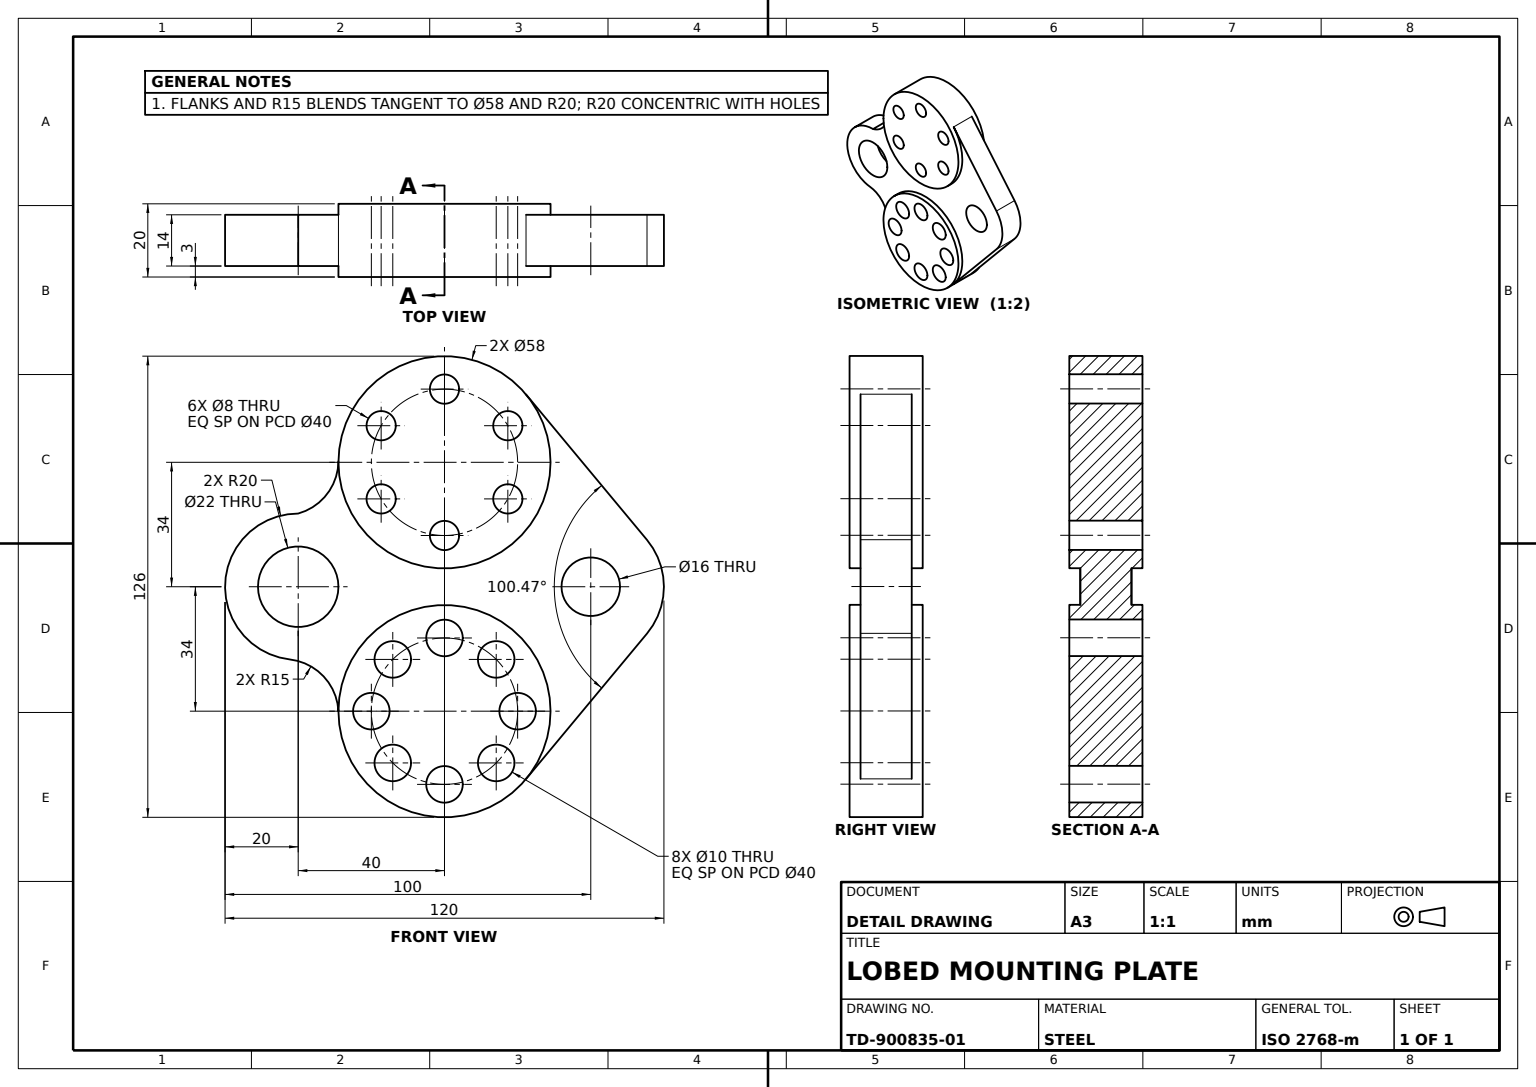
from build123d import *

# Parameters (mm, degrees)
TRI_LOBE_PLATE_PROFILE_R          = 29
TRI_LOBE_PLATE_PROFILE_R_2        = 5
LOBE_PADS_EXTRUDE_20MM_DEPTH      = 10
TRI_LOBE_PLATE_PROFILE_R_3        = 4
LOBE_PADS_EXTRUDE_20MM_2_DEPTH    = 10
SKETCH1_3_R                       = 8
SKETCH1_3_R_2                     = 11
CONNECTING_WEB_EXTRUDE_14MM_DEPTH = 7


with BuildPart() as part:
    # Tri-Lobe Plate Profile → Lobe Pads Extrude 20mm (new, symmetric)
    with BuildSketch(Plane.XY):
        Circle(TRI_LOBE_PLATE_PROFILE_R)
        with Locations((-14.142135624, 14.142135624)):
            Circle(TRI_LOBE_PLATE_PROFILE_R_2, mode=Mode.SUBTRACT)
        with Locations((-20, 0)):
            Circle(TRI_LOBE_PLATE_PROFILE_R_2, mode=Mode.SUBTRACT)
        with Locations((-14.142135624, -14.142135624)):
            Circle(TRI_LOBE_PLATE_PROFILE_R_2, mode=Mode.SUBTRACT)
        with Locations((0, -20)):
            Circle(TRI_LOBE_PLATE_PROFILE_R_2, mode=Mode.SUBTRACT)
        with Locations((14.142135624, -14.142135624)):
            Circle(TRI_LOBE_PLATE_PROFILE_R_2, mode=Mode.SUBTRACT)
        with Locations((20, 0)):
            Circle(TRI_LOBE_PLATE_PROFILE_R_2, mode=Mode.SUBTRACT)
        with Locations((14.142135624, 14.142135624)):
            Circle(TRI_LOBE_PLATE_PROFILE_R_2, mode=Mode.SUBTRACT)
        with Locations((0, 20)):
            Circle(TRI_LOBE_PLATE_PROFILE_R_2, mode=Mode.SUBTRACT)
    extrude(amount=LOBE_PADS_EXTRUDE_20MM_DEPTH, both=True)



with BuildPart() as body_2:
    # Tri-Lobe Plate Profile → Lobe Pads Extrude 20mm 2 (new, symmetric)
    with BuildSketch(Plane.XY):
        with Locations((0, -68)):
            Circle(TRI_LOBE_PLATE_PROFILE_R)
        with Locations((17.320508076, -78)):
            Circle(TRI_LOBE_PLATE_PROFILE_R_3, mode=Mode.SUBTRACT)
        with Locations((17.320508076, -58)):
            Circle(TRI_LOBE_PLATE_PROFILE_R_3, mode=Mode.SUBTRACT)
        with Locations((0, -48)):
            Circle(TRI_LOBE_PLATE_PROFILE_R_3, mode=Mode.SUBTRACT)
        with Locations((-17.320508076, -58)):
            Circle(TRI_LOBE_PLATE_PROFILE_R_3, mode=Mode.SUBTRACT)
        with Locations((-17.320508076, -78)):
            Circle(TRI_LOBE_PLATE_PROFILE_R_3, mode=Mode.SUBTRACT)
        with Locations((0, -88)):
            Circle(TRI_LOBE_PLATE_PROFILE_R_3, mode=Mode.SUBTRACT)
    extrude(amount=LOBE_PADS_EXTRUDE_20MM_2_DEPTH, both=True)


with BuildPart() as part_1:
    add(part.part)

    add(body_2.part)  # Connecting Web Extrude 14mm merges body 2
    # Sketch1_3 → Connecting Web Extrude 14mm (add, symmetric)
    with BuildSketch(Plane.XY):
        with BuildLine():
            Line((-22.291841993, 18.549225875), (-55.373684133, -21.207430431))
            ThreePointArc((-55.373684133, -21.207430431), (-60, -34), (-55.373684133, -46.792569569))
            Line((-55.373684133, -46.792569569), (-22.291841993, -86.549225875))
            ThreePointArc((-22.291841993, -86.549225875), (-9.862468813, -40.728555064), (29, -68))
            ThreePointArc((29, -68), (28.999608095, -68.150765842), (28.99843239, -68.301527609))
            ThreePointArc((28.99843239, -68.301527609), (32.108419422, -59.311623745), (40, -54))
            ThreePointArc((40, -54), (59.967539964, -35.139011754), (42.274326272, -14.129734778))
            ThreePointArc((42.274326272, -14.129734778), (33.047712472, -9.497553742), (29, 0))
            ThreePointArc((29, 0), (-9.862468813, -27.271444936), (-22.291841993, 18.549225875))
        make_face()
        with Locations((-40, -34)):
            Circle(SKETCH1_3_R, mode=Mode.SUBTRACT)
        with Locations((40, -34)):
            Circle(SKETCH1_3_R_2, mode=Mode.SUBTRACT)
    extrude(amount=CONNECTING_WEB_EXTRUDE_14MM_DEPTH, both=True)


solid = part_1.part
